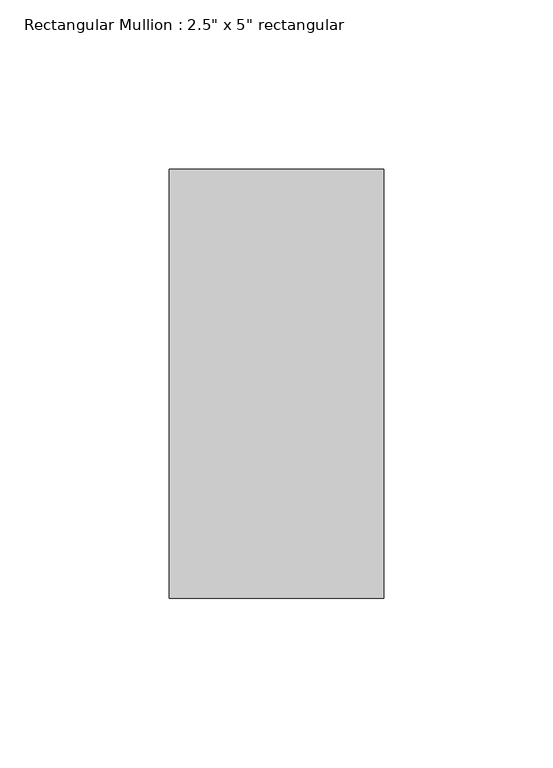
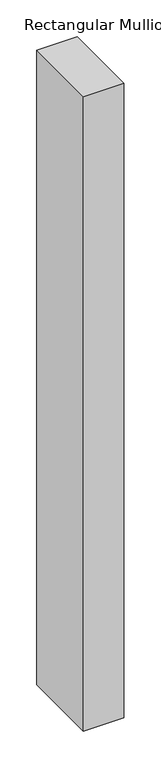
"""IFC4 building model written with IfcOpenShell, lengths in millimetres: member geometry."""

from ifc_helpers import new_model, si_unit, frame, origin, place, context, project, spatial, polyline, outline, extrude, source, transform, mapped, element, save


def member_7fa39cca(model_context):
    return source(origin(), model_context, "Body", "SweptSolid", [
        extrude(outline(polyline([(0.0, 63.5), (0.0, -63.5), (-63.5, -63.5), (-63.5, 63.5), (0.0, 63.5)])), frame((0.0, 0.0, -1054.1), z_axis=(0.0, 0.0, 1.0), x_axis=(1.0, 0.0, 0.0)), (0.0, 0.0, 1.0), 1054.1),
    ])


if __name__ == "__main__":
    model = new_model("IFC4")
    model_context = context("Model", 3, world=origin())
    ifc_project = project(units=[si_unit("LENGTHUNIT", "METRE", prefix="MILLI")], contexts=[model_context])
    site = spatial("IfcSite", under=ifc_project)
    building = spatial("IfcBuilding", under=site)
    placement = place(None, origin())
    member_shape = member_7fa39cca(model_context)
    element("IfcMember", 1, ObjectType="Rectangular Mullion : 2.5\" x 5\" rectangular", at=placement, inside=building, context=model_context, shape_type="MappedRepresentation", body=[
        mapped(member_shape, transform((0.0, 0.0, 0.0), x_axis=(1.0, 0.0, 0.0), y_axis=(0.0, 1.0, 0.0), z_axis=(0.0, 0.0, 1.0))),
    ])
    save(model, "model.ifc")

# Revit data of these elements
# Type "Rectangular Mullion : 2.5\" x 5\" rectangular"
#   built-in parameter 1007304 = 0.416667 (stored number, unit not read)
#   built-in parameter 1007301 = 0.104167 (stored number, unit not read)
#   built-in parameter 1007300 = 0.104167 (stored number, unit not read)
# Element 1 (IfcMember, "Rectangular Mullion : 2.5\" x 5\" rectangular")
#   Materials on its faces: "Aluminum"
# Materials
#   "Aluminum": class "Metal", colour RGB 247 247 247, transparency 0, Description = "Aluminum 6061", Cost = 0
